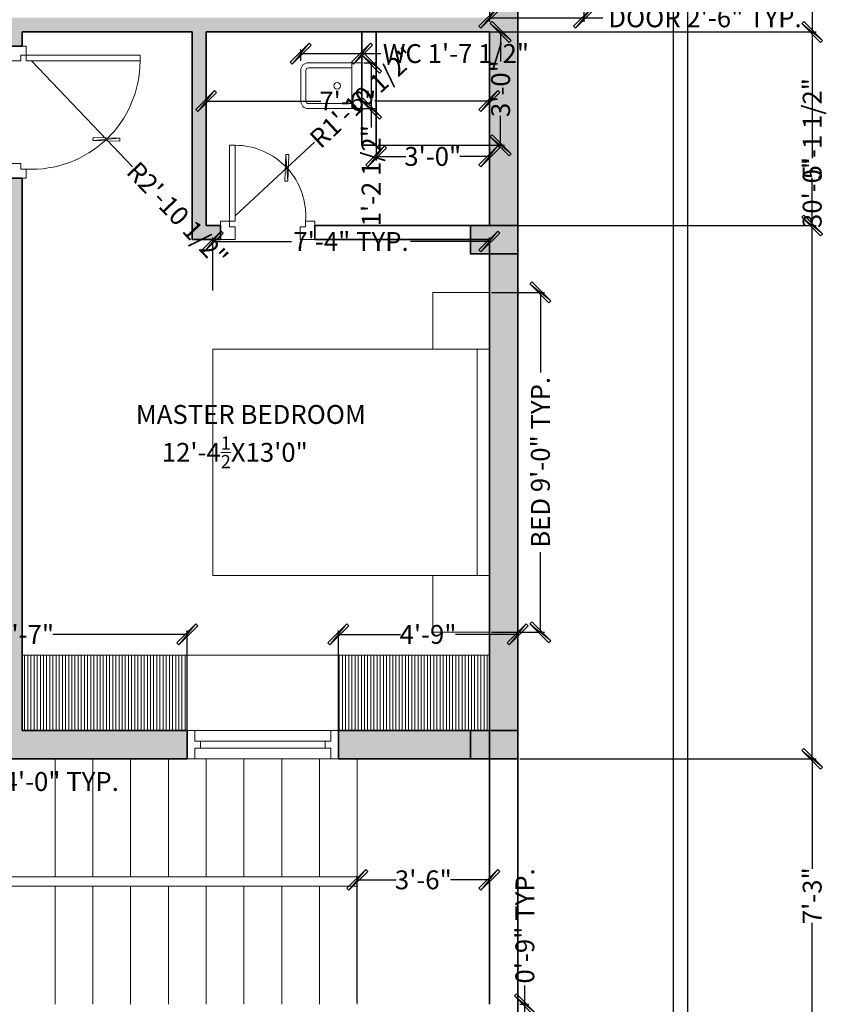
# Model space of a CAD drawing. Units: inches. Extents: x 1018 to 2596, y 723 to 1501.
# Tile 4 of 6: x 1425 to 1686, y 916 to 1229. Entities that reach past the tile are written whole.
import ezdxf

# ---------------------------------------------------------------- set-up
doc = ezdxf.new("R2010")
doc.units = ezdxf.units.IN
doc.layers.get('Defpoints').update_dxf_attribs({"lineweight": 0})
for name, color, linetype, lineweight in [('A-ANNO-DIMS', 2, 'Continuous', 13), ('A-AREA-IDEN', 7, 'Continuous', 18), ('A-COLS', 7, 'Continuous', 35), ('A-DOOR', 4, 'Continuous', 18), ('A-FLOR-CASE', 8, 'Continuous', 18), ('A-FLOR-CASE-PATT', 9, 'Continuous', 9), ('A-FLOR-FIXT', 9, 'Continuous', 18), ('A-FLOR-STRS', 7, 'Continuous', 18), ('A-FURN', 8, 'Continuous', 13), ('A-WALL', 7, 'Continuous', 35), ('A-WINDOW', 4, 'Continuous', 13), ('C-PROP', 7, 'Continuous', 25)]:
    doc.layers.add(name, color=color, linetype=linetype, lineweight=lineweight)
doc.layers.add('A-WALL-PATT', color=9, linetype='Continuous', lineweight=9, true_color=0xc7c8ca)
doc.styles.get("Standard").update_dxf_attribs({"font": 'arial.ttf'})
doc.dimstyles.new('saketh', dxfattribs={"dimtxt": 6, "dimasz": 6, "dimexe": 1.25, "dimexo": 0.625, "dimtad": 0, "dimdec": 1, "dimlunit": 4, "dimtxsty": 'Standard', "dimblk": 'ARCHTICK', "dimcen": 2.5, "dimclrd": 256, "dimclre": 1, "dimadec": 0, "dimazin": 0, "dimtfac": 1, "dimtdec": 1, "dimtmove": 0, "dimatfit": 3, "dimldrblk": 'ARCHTICK', "dimfxl": 1, "dimtolj": 1, "dimarcsym": 0})

# ---------------------------------------------------------------- blocks, each defined once
blk = doc.blocks.new('3 6 2')
at = {"layer": 'A-DOOR'}
for points in [[(-36.75, 5.83), (-36.75, 42), (-35, 42), (-35, 5.83)], [(-36.75, 4.08), (-35, 4.08), (-35, 0), (-39.67, 0), (-39.67, 5.83), (-36.75, 5.83)], [(-0.58, 5.83), (-0.58, 4.08), (-2.33, 4.08), (-2.33, 0), (2.33, 0), (2.33, 5.83)]]:
    blk.add_lwpolyline(points, close=True, dxfattribs=at)
at = {"layer": 'A-DOOR', "ltscale": 0.1}
blk.add_arc((-35, 7.54), 34.46, 357.1595, 90, dxfattribs=at)
blk = doc.blocks.new('2 feet 6 inch door')
at = {"layer": 'A-DOOR'}
for points in [[(2.92, 5.83), (2.92, 30), (4.67, 30), (4.67, 5.83)], [(2.92, 4.08), (4.67, 4.08), (4.67, 0), (0, 0), (0, 5.83), (2.92, 5.83)], [(27.08, 5.83), (27.08, 4.08), (25.33, 4.08), (25.33, 0), (30, 0), (30, 5.83)]]:
    blk.add_lwpolyline(points, close=True, dxfattribs=at)
at = {"layer": 'A-DOOR', "ltscale": 0.1}
blk.add_arc((4.67, 7.52), 22.48, 355.6972, 90, dxfattribs=at)
blk = doc.blocks.new('BED')
at = {"layer": 'A-FURN'}
for points in [[(1841.83, 1404.74), (1769.83, 1404.74), (1769.83, 1488.74), (1841.83, 1488.74)], [(1769.83, 1400.81), (1751.83, 1400.81), (1751.83, 1418.81), (1769.83, 1418.81)], [(1841.83, 1400.81), (1859.83, 1400.81), (1859.83, 1418.81), (1841.83, 1418.81)], [(1769.83, 1404.74), (1841.83, 1404.74), (1841.83, 1400.81), (1769.83, 1400.81)]]:
    blk.add_lwpolyline(points, close=True, dxfattribs=at)
blk = doc.blocks.new('WINDOW FRAME')
at = {"layer": 'A-WINDOW'}
for points in [[(4180.39, 4970.76), (4180.39, 4972.59), (4178.2, 4972.59), (4178.2, 4970.76)], [(4178.2, 4970.76), (4174.8, 4970.76), (4174.8, 4968.41), (4183.8, 4968.41), (4183.8, 4970.76), (4180.39, 4970.76)]]:
    blk.add_lwpolyline(points, dxfattribs=at)
blk = doc.blocks.new("4' window")
at = {"layer": 'A-WINDOW'}
for p, q in [((2.35, 9), (45.65, 9)), ((43.82, 5.59), (4.18, 5.59)), ((43.82, 3.41), (4.18, 3.41)), ((2.35, 0), (45.65, 0))]:
    blk.add_line(p, q, dxfattribs=at)
at = {"layer": 'A-WINDOW', "rotation": 270}
blk.add_blockref('WINDOW FRAME', (-4968.41, 4183.8), dxfattribs=at)
at = {"layer": 'A-WINDOW', "xscale": -1, "rotation": 90}
blk.add_blockref('WINDOW FRAME', (5016.41, 4183.8), dxfattribs=at)
blk = doc.blocks.new('WC')
at = {"layer": 'A-FURN'}
for p, q in [((0, 14.59), (-17.02, 14.59)), ((-3.24, 12.97), (-17.02, 12.97)), ((-3.24, 14.59), (-3.24, 0)), ((-19.45, 2.43), (-19.45, 12.16)), ((-17.83, 2.43), (-17.83, 12.16)), ((-3.24, 1.62), (-17.02, 1.62)), ((0, 0), (-17.02, 0))]:
    blk.add_line(p, q, dxfattribs=at)
blk.add_circle((-7.84, 7.3), 1.05, dxfattribs=at)
for centre, radius, start, end in [((-17.02, 12.16), 2.43, 90, 180), ((-17.02, 12.16), 0.811, 90, 180), ((-17.02, 2.43), 2.43, 180, 270), ((-17.02, 2.43), 0.811, 180, 270)]:
    blk.add_arc(centre, radius, start, end, dxfattribs=at)
blk = doc.blocks.new('COLUMN-15X9-IN')
h = blk.add_hatch(color=256)
h.dxf.hatch_style = 1
h.paths.add_polyline_path([(15, 0), (15, 9), (0, 9), (0, 0)])
blk.add_lwpolyline([(15, 9), (15, 0), (0, 0), (0, 9)], close=True)
blk = doc.blocks.new('_ArchTick')
for p, q in [((0.447, 0.553), (-0.553, -0.447)), ((0.553, 0.447), (0.447, 0.553)), ((-0.447, -0.553), (0.553, 0.447)), ((-0.553, -0.447), (-0.447, -0.553))]:
    blk.add_line(p, q)
mesh = blk.add_polyface()
corners = [(-0.447, -0.553), (0.447, 0.553), (-0.553, -0.447), (0.553, 0.447)]
mesh.append_faces([[corners[k] for k in face] for face in [(0, 1, 2), (1, 0, 3)]], dxfattribs={"vtx0": -1})
blk = doc.blocks.new('*D57')
at = {"layer": 'A-ANNO-DIMS', "color": 1, "lineweight": -2, "transparency": 16777216}
for p, q in [((1568.69, 906.1), (1568.69, 903.23)), ((1583.69, 906.1), (1583.69, 903.23))]:
    blk.add_line(p, q, dxfattribs=at)
at = {"layer": 'A-ANNO-DIMS', "lineweight": -2, "transparency": 16777216}
for p, q in [((1568.69, 904.48), (1583.69, 904.48)), ((1583.69, 904.48), (1589.69, 904.48))]:
    blk.add_line(p, q, dxfattribs=at)
at = {"layer": 'Defpoints', "color": 0, "transparency": 16777216}
for p in [(1568.69, 906.73), (1583.69, 906.73), (1583.69, 904.48)]:
    blk.add_point(p, dxfattribs=at)
at = {"layer": 'A-ANNO-DIMS', "lineweight": -2, "transparency": 16777216, "xscale": 6, "yscale": 6, "zscale": 6, "rotation": 180}
blk.add_blockref('_ArchTick', (1568.69, 904.48), dxfattribs=at)
at = {"layer": 'A-ANNO-DIMS', "lineweight": -2, "transparency": 16777216, "xscale": 6, "yscale": 6, "zscale": 6}
blk.add_blockref('_ArchTick', (1583.69, 904.48), dxfattribs=at)
at = {"layer": 'A-ANNO-DIMS', "color": 0, "transparency": 16777216, "insert": (1627.89, 904.48), "char_height": 6, "attachment_point": 5}
blk.add_mtext('\\A1;COLUMN 1\'-3" TYP.', dxfattribs=at)
blk = doc.blocks.new('*D58')
at = {"layer": 'A-ANNO-DIMS', "lineweight": -2, "transparency": 16777216}
for p, q in [((1585.94, 915.73), (1585.94, 921.73)), ((1585.94, 906.73), (1585.94, 915.73))]:
    blk.add_line(p, q, dxfattribs=at)
at = {"layer": 'A-ANNO-DIMS', "color": 1, "lineweight": -2, "transparency": 16777216}
for p, q in [((1584.31, 915.73), (1587.19, 915.73)), ((1584.31, 906.73), (1587.19, 906.73))]:
    blk.add_line(p, q, dxfattribs=at)
at = {"layer": 'Defpoints', "color": 0, "transparency": 16777216}
for p in [(1583.69, 915.73), (1585.94, 915.73), (1583.69, 906.73)]:
    blk.add_point(p, dxfattribs=at)
at = {"layer": 'A-ANNO-DIMS', "lineweight": -2, "transparency": 16777216, "xscale": 6, "yscale": 6, "zscale": 6}
for p, rotation in [((1585.94, 915.73), 90), ((1585.94, 906.73), 270)]:
    blk.add_blockref('_ArchTick', p, dxfattribs=dict(at, rotation=rotation))
at = {"layer": 'A-ANNO-DIMS', "color": 0, "transparency": 16777216, "insert": (1585.94, 940.64), "char_height": 6, "attachment_point": 5, "rotation": 90}
blk.add_mtext('\\A1;0\'-9" TYP.', dxfattribs=at)
blk = doc.blocks.new('*D61')
at = {"layer": 'A-ANNO-DIMS', "color": 1, "lineweight": -2, "transparency": 16777216}
for p, q in [((1574.69, 1233.1), (1574.69, 1227.98)), ((1604.69, 1233.1), (1604.69, 1227.98))]:
    blk.add_line(p, q, dxfattribs=at)
at = {"layer": 'A-ANNO-DIMS', "lineweight": -2, "transparency": 16777216}
for p, q in [((1574.69, 1229.23), (1604.69, 1229.23)), ((1604.69, 1229.23), (1610.69, 1229.23))]:
    blk.add_line(p, q, dxfattribs=at)
at = {"layer": 'Defpoints', "color": 0, "transparency": 16777216}
for p in [(1574.69, 1233.73), (1604.69, 1233.73), (1604.69, 1229.23)]:
    blk.add_point(p, dxfattribs=at)
at = {"layer": 'A-ANNO-DIMS', "lineweight": -2, "transparency": 16777216, "xscale": 6, "yscale": 6, "zscale": 6, "rotation": 180}
blk.add_blockref('_ArchTick', (1574.69, 1229.23), dxfattribs=at)
at = {"layer": 'A-ANNO-DIMS', "lineweight": -2, "transparency": 16777216, "xscale": 6, "yscale": 6, "zscale": 6}
blk.add_blockref('_ArchTick', (1604.69, 1229.23), dxfattribs=at)
at = {"layer": 'A-ANNO-DIMS', "color": 0, "transparency": 16777216, "insert": (1643.19, 1229.23), "char_height": 6, "attachment_point": 5}
blk.add_mtext('\\A1;DOOR 2\'-6" TYP.', dxfattribs=at)
blk = doc.blocks.new('*D65')
at = {"layer": 'A-ANNO-DIMS', "color": 1, "lineweight": -2, "transparency": 16777216}
for p, q in [((1575.31, 1141.96), (1592.14, 1141.96)), ((1575.31, 1033.96), (1592.14, 1033.96))]:
    blk.add_line(p, q, dxfattribs=at)
at = {"layer": 'A-ANNO-DIMS', "lineweight": -2, "transparency": 16777216}
for p, q in [((1590.89, 1141.96), (1590.89, 1116.52)), ((1590.89, 1033.96), (1590.89, 1059.4))]:
    blk.add_line(p, q, dxfattribs=at)
at = {"layer": 'Defpoints', "color": 0, "transparency": 16777216}
for p in [(1574.69, 1141.96), (1590.89, 1141.96), (1574.69, 1033.96)]:
    blk.add_point(p, dxfattribs=at)
at = {"layer": 'A-ANNO-DIMS', "lineweight": -2, "transparency": 16777216, "xscale": 6, "yscale": 6, "zscale": 6}
for p, rotation in [((1590.89, 1141.96), 90), ((1590.89, 1033.96), 270)]:
    blk.add_blockref('_ArchTick', p, dxfattribs=dict(at, rotation=rotation))
at = {"layer": 'A-ANNO-DIMS', "color": 0, "transparency": 16777216, "insert": (1590.89, 1087.96), "char_height": 6, "attachment_point": 5, "rotation": 90}
blk.add_mtext('\\A1;BED 9\'-0" TYP.', dxfattribs=at)
blk = doc.blocks.new('*D66')
at = {"layer": 'A-ANNO-DIMS', "color": 1, "lineweight": -2, "transparency": 16777216}
for p, q in [((1486.76, 1142.58), (1486.76, 1159.41)), ((1574.69, 1142.58), (1574.69, 1159.41))]:
    blk.add_line(p, q, dxfattribs=at)
at = {"layer": 'A-ANNO-DIMS', "lineweight": -2, "transparency": 16777216}
for p, q in [((1486.76, 1158.16), (1511.84, 1158.16)), ((1574.69, 1158.16), (1549.61, 1158.16))]:
    blk.add_line(p, q, dxfattribs=at)
at = {"layer": 'Defpoints', "color": 0, "transparency": 16777216}
for p in [(1486.76, 1158.16), (1486.76, 1141.96), (1574.69, 1141.96)]:
    blk.add_point(p, dxfattribs=at)
at = {"layer": 'A-ANNO-DIMS', "lineweight": -2, "transparency": 16777216, "xscale": 6, "yscale": 6, "zscale": 6, "rotation": 180}
blk.add_blockref('_ArchTick', (1486.76, 1158.16), dxfattribs=at)
at = {"layer": 'A-ANNO-DIMS', "lineweight": -2, "transparency": 16777216, "xscale": 6, "yscale": 6, "zscale": 6}
blk.add_blockref('_ArchTick', (1574.69, 1158.16), dxfattribs=at)
at = {"layer": 'A-ANNO-DIMS', "color": 0, "transparency": 16777216, "insert": (1530.72, 1158.16), "char_height": 6, "attachment_point": 5}
blk.add_mtext('\\A1;7\'-4" TYP.', dxfattribs=at)
blk = doc.blocks.new('*D67')
at = {"layer": 'A-ANNO-DIMS', "color": 1, "lineweight": -2, "transparency": 16777216}
for p, q in [((1327.94, 993.1), (1327.94, 985.28)), ((1375.94, 993.1), (1375.94, 985.28))]:
    blk.add_line(p, q, dxfattribs=at)
at = {"layer": 'A-ANNO-DIMS', "lineweight": -2, "transparency": 16777216}
for p, q in [((1327.94, 986.53), (1375.94, 986.53)), ((1375.94, 986.53), (1381.94, 986.53))]:
    blk.add_line(p, q, dxfattribs=at)
at = {"layer": 'Defpoints', "color": 0, "transparency": 16777216}
for p in [(1327.94, 993.73), (1375.94, 993.73), (1375.94, 986.53)]:
    blk.add_point(p, dxfattribs=at)
at = {"layer": 'A-ANNO-DIMS', "lineweight": -2, "transparency": 16777216, "xscale": 6, "yscale": 6, "zscale": 6, "rotation": 180}
blk.add_blockref('_ArchTick', (1327.94, 986.53), dxfattribs=at)
at = {"layer": 'A-ANNO-DIMS', "lineweight": -2, "transparency": 16777216, "xscale": 6, "yscale": 6, "zscale": 6}
blk.add_blockref('_ArchTick', (1375.94, 986.53), dxfattribs=at)
at = {"layer": 'A-ANNO-DIMS', "color": 0, "transparency": 16777216, "insert": (1420.52, 986.53), "char_height": 6, "attachment_point": 5}
blk.add_mtext('\\A1;WINDOW 4\'-0" TYP.', dxfattribs=at)
blk = doc.blocks.new('*D77')
at = {"layer": 'A-ANNO-DIMS', "color": 1, "lineweight": -2, "transparency": 16777216}
for p, q in [((1514.73, 1215.58), (1514.73, 1219.12)), ((1534.19, 1215.58), (1534.19, 1219.12))]:
    blk.add_line(p, q, dxfattribs=at)
at = {"layer": 'A-ANNO-DIMS', "lineweight": -2, "transparency": 16777216}
for p, q in [((1514.73, 1217.87), (1534.19, 1217.87)), ((1534.19, 1217.87), (1540.19, 1217.87))]:
    blk.add_line(p, q, dxfattribs=at)
at = {"layer": 'Defpoints', "color": 0, "transparency": 16777216}
for p in [(1534.19, 1217.87), (1514.73, 1214.95), (1534.19, 1214.95)]:
    blk.add_point(p, dxfattribs=at)
at = {"layer": 'A-ANNO-DIMS', "lineweight": -2, "transparency": 16777216, "xscale": 6, "yscale": 6, "zscale": 6, "rotation": 180}
blk.add_blockref('_ArchTick', (1514.73, 1217.87), dxfattribs=at)
at = {"layer": 'A-ANNO-DIMS', "lineweight": -2, "transparency": 16777216, "xscale": 6, "yscale": 6, "zscale": 6}
blk.add_blockref('_ArchTick', (1534.19, 1217.87), dxfattribs=at)
at = {"layer": 'A-ANNO-DIMS', "color": 0, "transparency": 16777216, "insert": (1564.05, 1217.87), "char_height": 6, "attachment_point": 5}
blk.add_mtext('\\A1;WC 1\'-7 1/2"', dxfattribs=at)
blk = doc.blocks.new('*D78')
at = {"layer": 'A-ANNO-DIMS', "color": 1, "lineweight": -2, "transparency": 16777216}
for p, q in [((1534.81, 1214.95), (1538.35, 1214.95)), ((1534.81, 1200.36), (1538.35, 1200.36))]:
    blk.add_line(p, q, dxfattribs=at)
at = {"layer": 'A-ANNO-DIMS', "lineweight": -2, "transparency": 16777216}
for p, q in [((1537.1, 1214.95), (1537.1, 1200.36)), ((1537.1, 1200.36), (1537.1, 1194.36))]:
    blk.add_line(p, q, dxfattribs=at)
at = {"layer": 'Defpoints', "color": 0, "transparency": 16777216}
for p in [(1534.19, 1214.95), (1534.19, 1200.36), (1537.1, 1200.36)]:
    blk.add_point(p, dxfattribs=at)
at = {"layer": 'A-ANNO-DIMS', "lineweight": -2, "transparency": 16777216, "xscale": 6, "yscale": 6, "zscale": 6}
for p, rotation in [((1537.1, 1214.95), 90), ((1537.1, 1200.36), 270)]:
    blk.add_blockref('_ArchTick', p, dxfattribs=dict(at, rotation=rotation))
at = {"layer": 'A-ANNO-DIMS', "color": 0, "transparency": 16777216, "insert": (1537.1, 1179.05), "char_height": 6, "attachment_point": 5, "rotation": 90}
blk.add_mtext('\\A1;1\'-2 1/2"', dxfattribs=at)
blk = doc.blocks.new('*D80')
at = {"layer": 'A-ANNO-DIMS', "color": 1, "lineweight": -2, "transparency": 16777216}
for p, q in [((1584.31, 1353.73), (1678.49, 1353.73)), ((1584.31, 993.73), (1678.49, 993.73))]:
    blk.add_line(p, q, dxfattribs=at)
at = {"layer": 'A-ANNO-DIMS', "lineweight": -2, "transparency": 16777216}
for p, q in [((1677.24, 1353.73), (1677.24, 1184.65)), ((1677.24, 993.73), (1677.24, 1162.8))]:
    blk.add_line(p, q, dxfattribs=at)
at = {"layer": 'Defpoints', "color": 0, "transparency": 16777216}
for p in [(1583.69, 1353.73), (1677.24, 1353.73), (1583.69, 993.73)]:
    blk.add_point(p, dxfattribs=at)
at = {"layer": 'A-ANNO-DIMS', "lineweight": -2, "transparency": 16777216, "xscale": 6, "yscale": 6, "zscale": 6}
for p, rotation in [((1677.24, 1353.73), 90), ((1677.24, 993.73), 270)]:
    blk.add_blockref('_ArchTick', p, dxfattribs=dict(at, rotation=rotation))
at = {"layer": 'A-ANNO-DIMS', "color": 0, "transparency": 16777216, "insert": (1677.24, 1173.73), "char_height": 6, "attachment_point": 5, "rotation": 90}
blk.add_mtext('\\A1;30\'-0"', dxfattribs=at)
blk = doc.blocks.new('*D81')
at = {"layer": 'A-ANNO-DIMS', "color": 1, "lineweight": -2, "transparency": 16777216}
for p, q in [((1584.31, 993.73), (1678.49, 993.73)), ((1584.31, 906.73), (1678.49, 906.73))]:
    blk.add_line(p, q, dxfattribs=at)
at = {"layer": 'A-ANNO-DIMS', "lineweight": -2, "transparency": 16777216}
for p, q in [((1677.24, 993.73), (1677.24, 958.8)), ((1677.24, 906.73), (1677.24, 941.65))]:
    blk.add_line(p, q, dxfattribs=at)
at = {"layer": 'Defpoints', "color": 0, "transparency": 16777216}
for p in [(1583.69, 993.73), (1677.24, 993.73), (1583.69, 906.73)]:
    blk.add_point(p, dxfattribs=at)
at = {"layer": 'A-ANNO-DIMS', "lineweight": -2, "transparency": 16777216, "xscale": 6, "yscale": 6, "zscale": 6}
for p, rotation in [((1677.24, 993.73), 90), ((1677.24, 906.73), 270)]:
    blk.add_blockref('_ArchTick', p, dxfattribs=dict(at, rotation=rotation))
at = {"layer": 'A-ANNO-DIMS', "color": 0, "transparency": 16777216, "insert": (1677.24, 950.23), "char_height": 6, "attachment_point": 5, "rotation": 90}
blk.add_mtext('\\A1;7\'-3"', dxfattribs=at)
blk = doc.blocks.new('*D87')
at = {"layer": 'A-ANNO-DIMS', "color": 1, "lineweight": -2, "transparency": 16777216}
for p, q in [((1532.69, 916.35), (1532.69, 956.53)), ((1574.69, 916.35), (1574.69, 956.53))]:
    blk.add_line(p, q, dxfattribs=at)
at = {"layer": 'A-ANNO-DIMS', "lineweight": -2, "transparency": 16777216}
for p, q in [((1532.69, 955.28), (1545.09, 955.28)), ((1574.69, 955.28), (1562.28, 955.28))]:
    blk.add_line(p, q, dxfattribs=at)
at = {"layer": 'Defpoints', "color": 0, "transparency": 16777216}
for p in [(1574.69, 955.28), (1532.69, 915.73), (1574.69, 915.73)]:
    blk.add_point(p, dxfattribs=at)
at = {"layer": 'A-ANNO-DIMS', "lineweight": -2, "transparency": 16777216, "xscale": 6, "yscale": 6, "zscale": 6, "rotation": 180}
blk.add_blockref('_ArchTick', (1532.69, 955.28), dxfattribs=at)
at = {"layer": 'A-ANNO-DIMS', "lineweight": -2, "transparency": 16777216, "xscale": 6, "yscale": 6, "zscale": 6}
blk.add_blockref('_ArchTick', (1574.69, 955.28), dxfattribs=at)
at = {"layer": 'A-ANNO-DIMS', "color": 0, "transparency": 16777216, "insert": (1553.69, 955.28), "char_height": 6, "attachment_point": 5}
blk.add_mtext('\\A1;3\'-6"', dxfattribs=at)
blk = doc.blocks.new('*D89')
at = {"layer": 'A-ANNO-DIMS', "color": 1, "lineweight": -2, "transparency": 16777216}
for p, q in [((1375.94, 994.35), (1375.94, 1034.53)), ((1478.69, 994.35), (1478.69, 1034.53))]:
    blk.add_line(p, q, dxfattribs=at)
at = {"layer": 'A-ANNO-DIMS', "lineweight": -2, "transparency": 16777216}
for p, q in [((1375.94, 1033.28), (1418.71, 1033.28)), ((1478.69, 1033.28), (1435.92, 1033.28))]:
    blk.add_line(p, q, dxfattribs=at)
at = {"layer": 'Defpoints', "color": 0, "transparency": 16777216}
for p in [(1478.69, 1033.28), (1375.94, 993.73), (1478.69, 993.73)]:
    blk.add_point(p, dxfattribs=at)
at = {"layer": 'A-ANNO-DIMS', "lineweight": -2, "transparency": 16777216, "xscale": 6, "yscale": 6, "zscale": 6, "rotation": 180}
blk.add_blockref('_ArchTick', (1375.94, 1033.28), dxfattribs=at)
at = {"layer": 'A-ANNO-DIMS', "lineweight": -2, "transparency": 16777216, "xscale": 6, "yscale": 6, "zscale": 6}
blk.add_blockref('_ArchTick', (1478.69, 1033.28), dxfattribs=at)
at = {"layer": 'A-ANNO-DIMS', "color": 0, "transparency": 16777216, "insert": (1427.31, 1033.28), "char_height": 6, "attachment_point": 5}
blk.add_mtext('\\A1;8\'-7"', dxfattribs=at)
blk = doc.blocks.new('*D90')
at = {"layer": 'A-ANNO-DIMS', "color": 1, "lineweight": -2, "transparency": 16777216}
for p, q in [((1526.69, 994.35), (1526.69, 1034.53)), ((1583.69, 994.35), (1583.69, 1034.53))]:
    blk.add_line(p, q, dxfattribs=at)
at = {"layer": 'A-ANNO-DIMS', "lineweight": -2, "transparency": 16777216}
for p, q in [((1526.69, 1033.28), (1546.47, 1033.28)), ((1583.69, 1033.28), (1563.91, 1033.28))]:
    blk.add_line(p, q, dxfattribs=at)
at = {"layer": 'Defpoints', "color": 0, "transparency": 16777216}
for p in [(1583.69, 1033.28), (1526.69, 993.73), (1583.69, 993.73)]:
    blk.add_point(p, dxfattribs=at)
at = {"layer": 'A-ANNO-DIMS', "lineweight": -2, "transparency": 16777216, "xscale": 6, "yscale": 6, "zscale": 6, "rotation": 180}
blk.add_blockref('_ArchTick', (1526.69, 1033.28), dxfattribs=at)
at = {"layer": 'A-ANNO-DIMS', "lineweight": -2, "transparency": 16777216, "xscale": 6, "yscale": 6, "zscale": 6}
blk.add_blockref('_ArchTick', (1583.69, 1033.28), dxfattribs=at)
at = {"layer": 'A-ANNO-DIMS', "color": 0, "transparency": 16777216, "insert": (1555.19, 1033.28), "char_height": 6, "attachment_point": 5}
blk.add_mtext('\\A1;4\'-9"', dxfattribs=at)
blk = doc.blocks.new('*D93')
at = {"layer": 'A-ANNO-DIMS', "color": 1, "lineweight": -2, "transparency": 16777216}
for p, q in [((1484.69, 1163.85), (1484.69, 1204.03)), ((1574.69, 1163.85), (1574.69, 1204.03))]:
    blk.add_line(p, q, dxfattribs=at)
at = {"layer": 'A-ANNO-DIMS', "lineweight": -2, "transparency": 16777216}
for p, q in [((1484.69, 1202.78), (1521.11, 1202.78)), ((1574.69, 1202.78), (1538.26, 1202.78))]:
    blk.add_line(p, q, dxfattribs=at)
at = {"layer": 'Defpoints', "color": 0, "transparency": 16777216}
for p in [(1574.69, 1202.78), (1484.69, 1163.23), (1574.69, 1163.23)]:
    blk.add_point(p, dxfattribs=at)
at = {"layer": 'A-ANNO-DIMS', "lineweight": -2, "transparency": 16777216, "xscale": 6, "yscale": 6, "zscale": 6, "rotation": 180}
blk.add_blockref('_ArchTick', (1484.69, 1202.78), dxfattribs=at)
at = {"layer": 'A-ANNO-DIMS', "lineweight": -2, "transparency": 16777216, "xscale": 6, "yscale": 6, "zscale": 6}
blk.add_blockref('_ArchTick', (1574.69, 1202.78), dxfattribs=at)
at = {"layer": 'A-ANNO-DIMS', "color": 0, "transparency": 16777216, "insert": (1529.69, 1202.78), "char_height": 6, "attachment_point": 5}
blk.add_mtext('\\A1;7\'-6"', dxfattribs=at)
blk = doc.blocks.new('*D94')
at = {"layer": 'A-ANNO-DIMS', "color": 1, "lineweight": -2, "transparency": 16777216}
for p, q in [((1575.31, 1224.73), (1678.49, 1224.73)), ((1575.31, 1163.23), (1678.49, 1163.23))]:
    blk.add_line(p, q, dxfattribs=at)
at = {"layer": 'A-ANNO-DIMS', "lineweight": -2, "transparency": 16777216}
for p, q in [((1677.24, 1224.73), (1677.24, 1209.57)), ((1677.24, 1163.23), (1677.24, 1178.39))]:
    blk.add_line(p, q, dxfattribs=at)
at = {"layer": 'Defpoints', "color": 0, "transparency": 16777216}
for p in [(1574.69, 1224.73), (1677.24, 1224.73), (1574.69, 1163.23)]:
    blk.add_point(p, dxfattribs=at)
at = {"layer": 'A-ANNO-DIMS', "lineweight": -2, "transparency": 16777216, "xscale": 6, "yscale": 6, "zscale": 6}
for p, rotation in [((1677.24, 1224.73), 90), ((1677.24, 1163.23), 270)]:
    blk.add_blockref('_ArchTick', p, dxfattribs=dict(at, rotation=rotation))
at = {"layer": 'A-ANNO-DIMS', "color": 0, "transparency": 16777216, "insert": (1677.24, 1193.98), "char_height": 6, "attachment_point": 5, "rotation": 90}
blk.add_mtext('\\A1;5\'-1 1/2"', dxfattribs=at)
blk = doc.blocks.new('*D97')
at = {"layer": 'A-ANNO-DIMS', "color": 1, "lineweight": -2, "transparency": 16777216}
for p, q in [((1539.31, 1224.73), (1579.49, 1224.73)), ((1539.31, 1188.73), (1579.49, 1188.73))]:
    blk.add_line(p, q, dxfattribs=at)
at = {"layer": 'A-ANNO-DIMS', "lineweight": -2, "transparency": 16777216}
for p, q in [((1578.24, 1224.73), (1578.24, 1215.32)), ((1578.24, 1188.73), (1578.24, 1198.13))]:
    blk.add_line(p, q, dxfattribs=at)
at = {"layer": 'Defpoints', "color": 0, "transparency": 16777216}
for p in [(1538.69, 1224.73), (1538.69, 1188.73), (1578.24, 1188.73)]:
    blk.add_point(p, dxfattribs=at)
at = {"layer": 'A-ANNO-DIMS', "lineweight": -2, "transparency": 16777216, "xscale": 6, "yscale": 6, "zscale": 6}
for p, rotation in [((1578.24, 1224.73), 90), ((1578.24, 1188.73), 270)]:
    blk.add_blockref('_ArchTick', p, dxfattribs=dict(at, rotation=rotation))
at = {"layer": 'A-ANNO-DIMS', "color": 0, "transparency": 16777216, "insert": (1578.24, 1206.73), "char_height": 6, "attachment_point": 5, "rotation": 90}
blk.add_mtext('\\A1;3\'-0"', dxfattribs=at)
blk = doc.blocks.new('*D98')
at = {"layer": 'A-ANNO-DIMS', "color": 1, "lineweight": -2, "transparency": 16777216}
for p, q in [((1538.69, 1224.1), (1538.69, 1183.93)), ((1574.69, 1224.1), (1574.69, 1183.93))]:
    blk.add_line(p, q, dxfattribs=at)
at = {"layer": 'A-ANNO-DIMS', "lineweight": -2, "transparency": 16777216}
for p, q in [((1538.69, 1185.18), (1548.09, 1185.18)), ((1574.69, 1185.18), (1565.28, 1185.18))]:
    blk.add_line(p, q, dxfattribs=at)
at = {"layer": 'Defpoints', "color": 0, "transparency": 16777216}
for p in [(1538.69, 1224.73), (1574.69, 1224.73), (1538.69, 1185.18)]:
    blk.add_point(p, dxfattribs=at)
at = {"layer": 'A-ANNO-DIMS', "lineweight": -2, "transparency": 16777216, "xscale": 6, "yscale": 6, "zscale": 6}
for p, rotation in [((1538.69, 1185.18), 179.9999999999982), ((1574.69, 1185.18), 359.9999999999982)]:
    blk.add_blockref('_ArchTick', p, dxfattribs=dict(at, rotation=rotation))
at = {"layer": 'A-ANNO-DIMS', "color": 0, "transparency": 16777216, "insert": (1556.69, 1185.18), "char_height": 6, "attachment_point": 5}
blk.add_mtext('\\A1;3\'-0"', dxfattribs=at)
blk = doc.blocks.new('*D115')
at = {"layer": 'A-ANNO-DIMS', "lineweight": -2, "transparency": 16777216}
for p in [(1429.23, 1215.56), (1461.26, 1181.9)]:
    blk.add_line(p, (1452.98, 1190.6), dxfattribs=at)
at = {"layer": 'Defpoints', "color": 0, "transparency": 16777216}
for p in [(1429.23, 1215.56), (1452.98, 1190.6)]:
    blk.add_point(p, dxfattribs=at)
at = {"layer": 'A-ANNO-DIMS', "lineweight": -2, "transparency": 16777216, "xscale": 6, "yscale": 6, "zscale": 6, "rotation": 133.5801307155605}
blk.add_blockref('_ArchTick', (1452.98, 1190.6), dxfattribs=at)
at = {"layer": 'A-ANNO-DIMS', "color": 0, "transparency": 16777216, "insert": (1475.59, 1166.84), "char_height": 6, "attachment_point": 5, "rotation": 313.5801}
blk.add_mtext('\\A1;R2\'-10 1/2"', dxfattribs=at)
blk = doc.blocks.new('*D116')
at = {"layer": 'A-ANNO-DIMS', "lineweight": -2, "transparency": 16777216}
for p in [(1519.13, 1189.69), (1493.85, 1166.25)]:
    blk.add_line(p, (1510.33, 1181.53), dxfattribs=at)
at = {"layer": 'Defpoints', "color": 0, "transparency": 16777216}
for p in [(1510.33, 1181.53), (1493.85, 1166.25)]:
    blk.add_point(p, dxfattribs=at)
at = {"layer": 'A-ANNO-DIMS', "lineweight": -2, "transparency": 16777216, "xscale": 6, "yscale": 6, "zscale": 6, "rotation": 222.8479764725387}
blk.add_blockref('_ArchTick', (1510.33, 1181.53), dxfattribs=at)
at = {"layer": 'A-ANNO-DIMS', "color": 0, "transparency": 16777216, "insert": (1534.38, 1203.83), "char_height": 6, "attachment_point": 5, "rotation": 42.848}
blk.add_mtext('\\A1;R1\'-10 1/2"', dxfattribs=at)

msp = doc.modelspace()

# ---------------------------------------------------------------- hatches: boundary and pattern name
at = {"layer": 'A-FLOR-CASE-PATT'}
h = msp.add_hatch(dxfattribs=at)
h.set_pattern_fill('_USER', color=256, angle=90, pattern_type=0)
h.set_pattern_definition([(90, (0, 0), (-1, 1e-16), [])])
h.paths.add_polyline_path([(1478.69, 1002.73), (1478.69, 1026.73), (1426.19, 1026.73), (1426.19, 1002.73)])
h.paths.add_polyline_path([(1574.69, 1002.73), (1574.69, 1026.73), (1526.69, 1026.73), (1526.69, 1002.73)])
at = {"layer": 'A-WALL-PATT', "transparency": 33554539}
h = msp.add_hatch(color=256, dxfattribs=at)
h.dxf.hatch_style = 1
h.paths.add_polyline_path([(1359.46, 1344.73), (1359.46, 1353.73), (1322.14, 1353.73), (1322.14, 1348.16), (1322.14, 1344.73)])
h.paths.add_polyline_path([(1374.46, 1353.73), (1374.46, 1344.73), (1421.69, 1344.73), (1421.69, 1296.73), (1415.69, 1296.73), (1415.69, 1292.23), (1426.19, 1292.23), (1426.19, 1344.73), (1568.69, 1344.73), (1568.69, 1353.73)])
h.paths.add_polyline_path([(1257.69, 1344.73), (1274.14, 1344.73), (1274.14, 1353.73), (1157.69, 1353.73), (1157.69, 1344.73)])
h.paths.add_polyline_path([(1151.69, 1344.73), (1142.69, 1344.73), (1142.69, 1257.11), (1148.25, 1257.11), (1151.69, 1257.11)])
h.paths.add_polyline_path([(1142.69, 1163.23), (1151.69, 1163.23), (1151.69, 1221.11), (1142.69, 1221.11)])
h.paths.add_polyline_path([(1151.69, 1154.23), (1142.69, 1154.23), (1142.69, 993.73), (1219.19, 993.73), (1219.19, 999.29), (1219.19, 1002.73), (1151.69, 1002.73)])
h.paths.add_polyline_path([(1327.94, 993.73), (1327.94, 1002.73), (1277.69, 1002.73), (1277.69, 1158.73), (1283.22, 1158.73), (1283.22, 1163.23), (1273.19, 1163.23), (1268.69, 1163.23), (1268.69, 1158.73), (1273.19, 1158.73), (1273.19, 1002.73), (1255.19, 1002.73), (1255.19, 993.73)])
h.paths.add_polyline_path([(1426.19, 1002.73), (1426.19, 1178.23), (1421.69, 1178.23), (1421.69, 1163.23), (1374.46, 1163.23), (1374.46, 1158.73), (1421.69, 1158.73), (1421.69, 1002.73), (1375.94, 1002.73), (1375.94, 993.73), (1478.69, 993.73), (1478.69, 1002.73)])
h.paths.add_polyline_path([(1583.69, 1233.73), (1574.69, 1233.73), (1574.69, 1229.23), (1421.69, 1229.23), (1421.69, 1220.23), (1426.19, 1220.23), (1426.19, 1224.73), (1480.19, 1224.73), (1480.19, 1158.73), (1489.19, 1158.73), (1489.19, 1163.23), (1484.69, 1163.23), (1484.69, 1224.73), (1508.69, 1224.73), (1574.69, 1224.73), (1574.69, 1163.23), (1583.69, 1163.23)])
h.paths.add_polyline_path([(1574.69, 1263.73), (1580.52, 1263.73), (1583.69, 1263.73), (1583.69, 1344.73), (1574.69, 1344.73)])
h.paths.add_polyline_path([(1583.69, 1154.23), (1574.69, 1154.23), (1574.69, 1002.73), (1583.69, 1002.73)])
h.paths.add_polyline_path([(1568.69, 993.73), (1568.69, 1002.73), (1526.69, 1002.73), (1526.69, 993.73)])
h.paths.add_polyline_path([(1359.46, 1158.73), (1359.46, 1163.23), (1325.22, 1163.23), (1325.22, 1158.73)])
h.paths.add_polyline_path([(1232.69, 1158.73), (1232.69, 1163.23), (1157.69, 1163.23), (1157.69, 1158.73)])

# ---------------------------------------------------------------- linework, layer by layer
at = {"layer": 'A-FLOR-CASE'}
for p, q in [((1574.69, 1026.73), (1426.19, 1026.73)), ((1478.69, 1002.73), (1478.69, 1026.73)), ((1526.69, 1002.73), (1526.69, 1026.73))]:
    msp.add_line(p, q, dxfattribs=at)
at = {"layer": 'A-FLOR-STRS'}
for p, q in [((1436.69, 993.73), (1436.69, 956.23)), ((1448.69, 993.73), (1448.69, 956.23)), ((1460.69, 993.73), (1460.69, 956.23)), ((1472.69, 993.73), (1472.69, 956.23)), ((1484.69, 993.73), (1484.69, 956.23)), ((1496.69, 993.73), (1496.69, 956.23)), ((1508.69, 993.73), (1508.69, 956.23)), ((1520.69, 993.73), (1520.69, 956.23)), ((1532.69, 993.73), (1532.69, 915.73)), ((1532.69, 956.23), (1400.69, 956.23)), ((1532.69, 953.23), (1400.69, 953.23)), ((1436.69, 953.23), (1436.69, 915.73)), ((1448.69, 953.23), (1448.69, 915.73)), ((1460.69, 953.23), (1460.69, 915.73)), ((1472.69, 953.23), (1472.69, 915.73)), ((1484.69, 953.23), (1484.69, 915.73)), ((1496.69, 953.23), (1496.69, 915.73)), ((1508.69, 953.23), (1508.69, 915.73)), ((1520.69, 953.23), (1520.69, 915.73))]:
    msp.add_line(p, q, dxfattribs=at)
at = {"layer": 'A-WALL'}
for p, q in [((1583.69, 1233.73), (1583.69, 906.73)), ((1426.19, 1224.73), (1480.19, 1224.73)), ((1426.19, 1224.73), (1426.19, 1220.23)), ((1480.19, 1224.73), (1480.19, 1158.73)), ((1484.69, 1224.73), (1484.69, 1163.23)), ((1484.69, 1224.73), (1574.69, 1224.73)), ((1534.19, 1224.73), (1534.19, 1188.73)), ((1538.69, 1224.73), (1538.69, 1188.73)), ((1574.69, 1224.73), (1574.69, 1163.23)), ((1426.19, 1220.23), (1421.69, 1220.23)), ((1534.19, 1188.73), (1538.69, 1188.73)), ((1426.19, 1178.23), (1421.69, 1178.23)), ((1426.19, 1178.23), (1426.19, 1002.73)), ((1489.19, 1163.23), (1484.69, 1163.23)), ((1489.19, 1163.23), (1489.19, 1158.73)), ((1574.69, 1163.23), (1519.19, 1163.23)), ((1519.19, 1163.23), (1519.19, 1158.73)), ((1489.19, 1158.73), (1480.19, 1158.73)), ((1574.69, 1158.73), (1519.19, 1158.73)), ((1574.69, 1158.73), (1574.69, 915.73)), ((1478.69, 1002.73), (1426.19, 1002.73)), ((1478.69, 1002.73), (1478.69, 993.73)), ((1574.69, 1002.73), (1526.69, 1002.73)), ((1526.69, 1002.73), (1526.69, 993.73)), ((1478.69, 993.73), (1375.94, 993.73)), ((1574.69, 993.73), (1526.69, 993.73))]:
    msp.add_line(p, q, dxfattribs=at)
at = {"layer": 'C-PROP'}
for points in [[(1405.19, 726.73), (1637.69, 726.73), (1637.69, 1473.73), (1052.69, 1473.73), (1052.69, 726.73), (1285.19, 726.73)], [(1405.19, 731.23), (1633.19, 731.23), (1633.19, 1469.23), (1057.19, 1469.23), (1057.19, 731.23), (1285.19, 731.23)]]:
    msp.add_lwpolyline(points, dxfattribs=at)

# ---------------------------------------------------------------- block references
at = {"layer": 'A-COLS'}
for p in [(1568.69, 1154.22), (1568.69, 993.73)]:
    msp.add_blockref('COLUMN-15X9-IN', p, dxfattribs=at)
at = {"layer": 'A-DOOR', "rotation": 270}
msp.add_blockref('3 6 2', (1421.69, 1180.56), dxfattribs=at)
at = {"layer": 'A-DOOR'}
msp.add_blockref('2 feet 6 inch door', (1489.19, 1158.73), dxfattribs=at)
at = {"layer": 'A-FLOR-FIXT', "xscale": -1, "rotation": 180}
msp.add_blockref('WC', (1534.19, 1214.95), dxfattribs=at)
at = {"layer": 'A-FURN', "rotation": 90}
msp.add_blockref('BED', (2975.5, -717.88), dxfattribs=at)
at = {"layer": 'A-WINDOW'}
msp.add_blockref("4' window", (1478.69, 993.73), dxfattribs=at)

# ---------------------------------------------------------------- texts
at = {"layer": 'A-AREA-IDEN', "insert": (1459.59, 1106.18), "char_height": 9, "attachment_point": 1}
msp.add_mtext_dynamic_manual_height_columns('\\A1; {\\H0.66667x;MASTER BEDROOM\\P      12\'-4\\H0.7x;\\S1/2;\\H1.42857x;X13\'0"}', width=129.8331, gutter_width=12.5, heights=[0], dxfattribs=at)

# ---------------------------------------------------------------- dimensions: what is measured, and where the dimension line sits
at = {"layer": 'A-ANNO-DIMS'}
for base, p1, p2, angle, picture, middle in [((1677.24, 1353.73), (1583.69, 993.73), (1583.69, 1353.73), 90, '*D80', (1677.24, 1173.73)), ((1578.24, 1188.73), (1538.69, 1224.73), (1538.69, 1188.73), 270, '*D97', (1578.24, 1206.73)), ((1677.24, 1224.73), (1574.69, 1163.23), (1574.69, 1224.73), 90, '*D94', (1677.24, 1193.98)), ((1538.69, 1185.18), (1574.69, 1224.73), (1538.69, 1224.73), 180, '*D98', (1556.69, 1185.18)), ((1537.1, 1200.36), (1534.19, 1214.95), (1534.19, 1200.36), 270, '*D78', (1537.1, 1179.05)), ((1478.686856, 1033.27536), (1375.936856, 993.725361), (1478.686856, 993.725359), 359.99999871, '*D89', (1427.311856, 1033.27536)), ((1583.69, 1033.28), (1526.69, 993.73), (1583.69, 993.73), 360, '*D90', (1555.19, 1033.28)), ((1677.24, 993.73), (1583.69, 906.73), (1583.69, 993.73), 90, '*D81', (1677.24, 950.23))]:
    dim = msp.add_linear_dim(base=base, p1=p1, p2=p2, angle=angle, dimstyle='saketh', override={"dimdec": 1, "dimlfac": 1, "dimrnd": 0, "dimzin": 1, "dimdsep": 46, "dimlunit": 4, "dimfrac": 2}, dxfattribs=at)
    dim.commit()
    dim.dimension.update_dxf_attribs({"geometry": picture, "text_midpoint": middle})
for base, p1, p2, text, picture, middle in [((1604.69, 1229.23), (1574.69, 1233.73), (1604.69, 1233.73), 'DOOR <> TYP.', '*D61', (1643.19, 1229.23)), ((1534.19, 1217.87), (1514.73, 1214.95), (1534.19, 1214.95), 'WC <>', '*D77', (1564.05, 1217.87)), ((1375.94, 986.53), (1327.94, 993.73), (1375.94, 993.73), 'WINDOW <> TYP.', '*D67', (1420.52, 986.53)), ((1583.69, 904.48), (1568.69, 906.73), (1583.69, 906.73), 'COLUMN <> TYP.', '*D57', (1627.89, 904.48))]:
    dim = msp.add_linear_dim(base=base, p1=p1, p2=p2, text=text, dimstyle='saketh', override={"dimdec": 1, "dimlfac": 1, "dimrnd": 0, "dimzin": 1, "dimdsep": 46, "dimlunit": 4, "dimfrac": 2}, dxfattribs=at)
    dim.commit()
    dim.dimension.update_dxf_attribs({"geometry": picture, "text_midpoint": middle})
for center, mpoint, picture, middle in [((1493.85, 1166.25), (1510.33, 1181.53), '*D116', (1534.38, 1203.83)), ((1429.23, 1215.56), (1452.98, 1190.6), '*D115', (1475.59, 1166.84))]:
    dim = msp.add_radius_dim(center=center, mpoint=mpoint, dimstyle='saketh', override={"dimdec": 1, "dimlfac": 1, "dimrnd": 0, "dimzin": 1, "dimdsep": 46, "dimlunit": 4, "dimfrac": 2}, dxfattribs=at)
    dim.commit()
    dim.dimension.update_dxf_attribs({"geometry": picture, "text_midpoint": middle})
for base, p1, p2, picture, middle in [((1574.69, 1202.78), (1484.69, 1163.23), (1574.69, 1163.23), '*D93', (1529.69, 1202.78)), ((1574.69, 955.28), (1532.69, 915.73), (1574.69, 915.73), '*D87', (1553.69, 955.28))]:
    dim = msp.add_linear_dim(base=base, p1=p1, p2=p2, dimstyle='saketh', override={"dimdec": 1, "dimlfac": 1, "dimrnd": 0, "dimzin": 1, "dimdsep": 46, "dimlunit": 4, "dimfrac": 2}, dxfattribs=at)
    dim.commit()
    dim.dimension.update_dxf_attribs({"geometry": picture, "text_midpoint": middle})
for base, p1, p2, angle, text, picture, middle in [((1486.76, 1158.16), (1574.69, 1141.96), (1486.76, 1141.96), 180, '<> TYP.', '*D66', (1530.72, 1158.16)), ((1590.89, 1141.96), (1574.69, 1033.96), (1574.69, 1141.96), 90, 'BED <> TYP.', '*D65', (1590.89, 1087.96)), ((1585.94, 915.73), (1583.69, 906.73), (1583.69, 915.73), 90, '<> TYP.', '*D58', (1585.94, 940.64))]:
    dim = msp.add_linear_dim(base=base, p1=p1, p2=p2, angle=angle, text=text, dimstyle='saketh', override={"dimdec": 1, "dimlfac": 1, "dimrnd": 0, "dimzin": 1, "dimdsep": 46, "dimlunit": 4, "dimfrac": 2}, dxfattribs=at)
    dim.commit()
    dim.dimension.update_dxf_attribs({"geometry": picture, "text_midpoint": middle})

doc.saveas('drawing.dxf')
